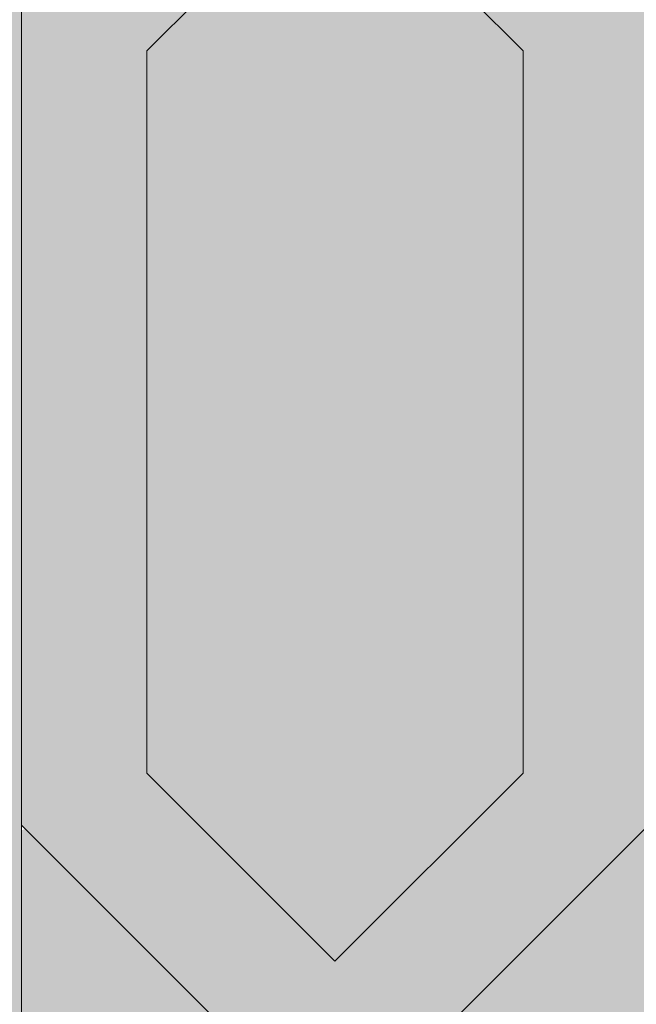
# Model space of a CAD drawing. Units: inches. Extents: x 844 to 2234, y 346 to 1084.
# Tile 78 of 93: x 1997.478 to 1998.732, y 704.51 to 706.514. Entities that reach past the tile are written whole.
import ezdxf

# ---------------------------------------------------------------- set-up
doc = ezdxf.new("R2010")
doc.units = ezdxf.units.IN
doc.header["$MEASUREMENT"] = 0
for name, color, linetype, lineweight in [('A-ANNO-DIMS', 2, 'Continuous', 18), ('furniture', 8, 'Continuous', 18), ('RA-AP-01$0$INT', 35, 'Continuous', 5)]:
    doc.layers.add(name, color=color, linetype=linetype, lineweight=lineweight)
doc.layers.add('RA-AP-01$0$FURN', color=3, linetype='Continuous')
doc.styles.get("Standard").update_dxf_attribs({"font": 'arial.ttf'})
doc.dimstyles.get("Standard").update_dxf_attribs({"dimtxt": 6, "dimasz": 3, "dimexe": 0.18, "dimexo": 0.0625, "dimgap": 0.09, "dimtad": 0, "dimtih": 1, "dimtoh": 1, "dimdec": 1, "dimzin": 0, "dimdsep": 46, "dimlunit": 3, "dimtxsty": 'Standard', "dimblk": 'ARCHTICK', "dimcen": 0.09, "dimadec": 0, "dimazin": 0, "dimtfac": 1, "dimtdec": 1, "dimtofl": 0, "dimtmove": 0, "dimatfit": 3, "dimfxl": 1, "dimtolj": 1, "dimtzin": 0, "dimarcsym": 0})

# ---------------------------------------------------------------- blocks, each defined once
blk = doc.blocks.new('A$C18D01794')
at = {"layer": 'RA-AP-01$0$INT'}
h = blk.add_hatch(color=256, dxfattribs=at)
h.paths.add_polyline_path([(4.355206456958071, -6.156712009588037), (4.355206456958071, -8.056712009588038), (5.455206456958072, -8.056712009588038), (5.455206456958072, -6.156712009588037)])
h.paths.add_polyline_path([(4.405206456958072, -8.006712009588039), (4.405206456958072, -6.206712009588038), (5.405206456958072, -6.206712009588038), (5.405206456958072, -8.006712009588039)], flags=16)
h = blk.add_hatch(color=256, dxfattribs=at)
h.paths.add_polyline_path([(4.505206456958071, -7.585498806127123), (4.46934859260189, -7.549640941759413), (4.505206456958071, -7.513783077414768), (4.505206456958071, -7.381963272220687), (4.469348592616735, -7.346105407867824), (4.505206456958071, -7.310247543514964), (4.505206456958071, -7.178427738324996), (4.469348592586679, -7.142569873965138), (4.505206456952245, -7.106712009588038), (4.476922185709333, -7.106712009588038), (4.455206456960671, -7.128427738343681), (4.433490728198047, -7.106712009588038), (4.405206456946033, -7.106712009588036), (4.441064321339216, -7.142569873969684), (4.40520645695807, -7.178427738362358), (4.405206456958072, -7.310247543472698), (4.441064321364728, -7.346105407867826), (4.40520645695807, -7.381963272262947), (4.40520645695807, -7.513783077378263), (4.441064321354429, -7.549640941786153), (4.405206456958072, -7.585498806170974), (4.405206456958072, -7.717318611286652), (4.441064321333084, -7.753176475673194), (4.405206456958072, -7.789034340036673), (4.405206456958072, -8.006712009588039), (4.644348592588106, -8.006712009588039), (4.680206456964639, -7.970854145211967), (4.716064321341165, -8.006712009588039), (4.869348592586113, -8.006712009588039), (4.905206456964143, -7.970854145210465), (4.941064321342174, -8.006712009588039), (5.094348592587118, -8.006712009588037), (5.130206456963649, -7.970854145211967), (5.166064321340178, -8.006712009588039), (5.405206456958072, -8.006712009588039), (5.405206456958072, -7.789034340024526), (5.369348592595202, -7.753176475673196), (5.40520645695807, -7.717318611298797), (5.40520645695807, -7.585498806158829), (5.369348592573859, -7.549640941786151), (5.40520645695807, -7.51378307739041), (5.40520645695807, -7.381963272250803), (5.36934859256356, -7.346105407867824), (5.405206456958072, -7.310247543484846), (5.405206456958072, -7.178427738350217), (5.369348592589068, -7.142569873969682), (5.405206456982249, -7.106712009588038), (5.376922185730244, -7.106712009588038), (5.355206456967613, -7.128427738343679), (5.333490728218955, -7.10671200958804), (5.305206456976043, -7.106712009588042), (5.341064321341609, -7.142569873965136), (5.305206456958072, -7.178427738337141), (5.305206456958072, -7.310247543502816), (5.34106432131155, -7.346105407867824), (5.305206456958072, -7.381963272232832), (5.30520645695807, -7.513783077402624), (5.341064321326395, -7.549640941759413), (5.305206456958072, -7.585498806139263), (5.305206456958072, -7.717318611299605), (5.341064321347738, -7.753176475677737), (5.305206456958072, -7.78903434007894), (5.30520645695807, -7.906712009588039), (5.166064321336834, -7.906712009588039), (5.130206456963647, -7.942569873961684), (5.094348592590464, -7.906712009588039), (4.941064321338827, -7.906712009588041), (4.905206456964145, -7.942569873963183), (4.869348592589459, -7.906712009588039), (4.716064321337822, -7.906712009588041), (4.680206456964641, -7.942569873961684), (4.644348592591453, -7.906712009588039), (4.505206456958071, -7.906712009588039), (4.505206456958071, -7.789034340066795), (4.469348592580545, -7.753176475677738), (4.505206456958071, -7.717318611311748)])
h.paths.add_polyline_path([(4.485206456974132, -7.709034340046354), (4.45520645695909, -7.739034340051736), (4.425206456974128, -7.709034340057131), (4.425206456993394, -7.593783077384998), (4.45520645699153, -7.563783077396511), (4.485206456993396, -7.593783077408017)], flags=16)
h.paths.add_polyline_path([(4.455206456954537, -7.767318611299197), (4.485206456958242, -7.797318611312542), (4.48520645695951, -7.912569873958716), (4.45520645695415, -7.942569873954422), (4.425206456957888, -7.912569873967813), (4.425206456957888, -7.797318611286197)], flags=16)
h.paths.add_polyline_path([(4.455206456964794, -7.535498806149051), (4.42520645696469, -7.5054988061393), (4.425206456983954, -7.390247543486406), (4.455206456990734, -7.360247543489279), (4.485206456983953, -7.39024754349214), (4.485206456964687, -7.505498806158811)], flags=16)
h.paths.add_polyline_path([(4.499348592588947, -7.926712009585049), (4.636064321340932, -7.926712009585049), (4.666064321342317, -7.956712009586821), (4.636064321343707, -7.986712009585048), (4.499348592575121, -7.986712009585048), (4.469348592591685, -7.956712009591957)], flags=16)
h.paths.add_polyline_path([(4.425206456957888, -7.940854145195974), (4.471064321332215, -7.986712009585049), (4.425206456957888, -7.986712009585049)], flags=16)
h.paths.add_polyline_path([(4.455206456990734, -7.331963272246367), (4.425206456989053, -7.301963272254337), (4.425206456969784, -7.186712009596224), (4.455206456965226, -7.156712009591144), (4.485206456969787, -7.186712009586051), (4.485206456989053, -7.301963272238404)], flags=16)
h.paths.add_polyline_path([(4.72434859258714, -7.926712009586255), (4.861064321340141, -7.926712009586248), (4.891064321340324, -7.956712009586823), (4.861064321340513, -7.986712009586252), (4.724348592586768, -7.986712009586252), (4.694348592586956, -7.956712009586821)], flags=16)
h.paths.add_polyline_path([(4.919348592587961, -7.956712009586821), (4.949348592588145, -7.92671200958625), (5.08606432134115, -7.926712009586253), (5.116064321341327, -7.956712009586823), (5.086064321341519, -7.986712009586252), (4.949348592587774, -7.986712009586252)], flags=16)
h.paths.add_polyline_path([(5.144348592585967, -7.956712009586823), (5.174348592587358, -7.926712009585049), (5.311064321339338, -7.926712009585049), (5.3410643213366, -7.956712009591957), (5.311064321353163, -7.986712009585048), (5.174348592584576, -7.986712009585048)], flags=16)
h.paths.add_polyline_path([(5.32520645693489, -7.593783077408021), (5.355206456936755, -7.563783077396511), (5.385206456934894, -7.593783077384998), (5.38520645695416, -7.709034340057128), (5.355206456969194, -7.739034340051736), (5.325206456954153, -7.709034340046352)], flags=16)
h.paths.add_polyline_path([(5.325206456970042, -7.797318611312542), (5.355206456973747, -7.767318611299197), (5.385206456970398, -7.7973186112862), (5.385206456970398, -7.912569873967816), (5.355206456974136, -7.942569873954422), (5.325206456968778, -7.912569873958716)], flags=16)
h.paths.add_polyline_path([(5.325206456963599, -7.505498806158811), (5.325206456944333, -7.39024754349214), (5.355206456937552, -7.360247543489279), (5.385206456944332, -7.39024754348641), (5.385206456963596, -7.505498806139303), (5.355206456963492, -7.53549880614905)], flags=16)
h.paths.add_polyline_path([(5.32520645693923, -7.301963272238403), (5.3252064569585, -7.186712009586051), (5.355206456963062, -7.156712009591142), (5.3852064569585, -7.186712009596224), (5.385206456939234, -7.301963272254338), (5.355206456937552, -7.331963272246369)], flags=16)
h.paths.add_polyline_path([(5.339348592596071, -7.986712009585048), (5.385206456970398, -7.940854145195972), (5.385206456970396, -7.986712009585048)], flags=16)
h = blk.add_hatch(color=256, dxfattribs=at)
h.paths.add_polyline_path([(4.469348592586677, -7.142569873965136), (4.505206456958073, -7.178427738324996), (4.505206456958071, -7.106712009582215)])
h.paths.add_polyline_path([(4.455206456960671, -7.128427738343681), (4.476922185709333, -7.106712009588038), (4.433490728198045, -7.106712009588038)])
h.paths.add_polyline_path([(4.405206456958073, -7.178427738362358), (4.441064321339218, -7.142569873969684), (4.40520645695807, -7.106712009600073)])
h.paths.add_polyline_path([(4.425206456989053, -7.301963272254335), (4.455206456990736, -7.331963272246371), (4.485206456989055, -7.301963272238399), (4.48520645696979, -7.186712009586054), (4.455206456965227, -7.15671200959114), (4.425206456969784, -7.186712009596224)])
h.paths.add_polyline_path([(4.505206456958073, -7.381963272220689), (4.505206456958071, -7.310247543514961), (4.469348592616738, -7.346105407867826)])
h.paths.add_polyline_path([(4.425206456964688, -7.5054988061393), (4.455206456964794, -7.535498806149051), (4.485206456964689, -7.505498806158811), (4.485206456983951, -7.390247543492138), (4.455206456990736, -7.360247543489277), (4.425206456983956, -7.39024754348641)])
h.paths.add_polyline_path([(4.425206456974126, -7.709034340057128), (4.455206456959092, -7.739034340051736), (4.485206456974132, -7.709034340046356), (4.485206456993396, -7.593783077408017), (4.45520645699153, -7.563783077396511), (4.425206456993394, -7.593783077384999)])
h.paths.add_polyline_path([(4.46934859260189, -7.549640941759415), (4.505206456958071, -7.585498806127123), (4.505206456958073, -7.513783077414766)])
h.paths.add_polyline_path([(4.405206456958073, -7.585498806170972), (4.441064321354427, -7.549640941786151), (4.405206456958072, -7.513783077378263)])
h.paths.add_polyline_path([(4.405206456958072, -7.789034340036673), (4.441064321333084, -7.753176475673194), (4.405206456958072, -7.71731861128665)])
h.paths.add_polyline_path([(4.469348592580547, -7.75317647567774), (4.505206456958071, -7.789034340066795), (4.505206456958071, -7.717318611311744)])
h.paths.add_polyline_path([(4.425206456957888, -7.912569873967814), (4.45520645695415, -7.942569873954422), (4.485206456959507, -7.912569873958718), (4.48520645695824, -7.797318611312542), (4.455206456954537, -7.767318611299197), (4.425206456957888, -7.797318611286202)])
h.paths.add_polyline_path([(4.425206456957888, -7.986712009585049), (4.471064321332215, -7.986712009585049), (4.425206456957888, -7.940854145195972)])
h.paths.add_polyline_path([(4.499348592575121, -7.986712009585048), (4.636064321343707, -7.986712009585049), (4.666064321342317, -7.956712009586823), (4.636064321340932, -7.926712009585049), (4.499348592588945, -7.926712009585049), (4.469348592591685, -7.95671200959196)])
h.paths.add_polyline_path([(4.680206456964641, -7.942569873961684), (4.716064321337824, -7.906712009588039), (4.644348592591454, -7.906712009588039)])
h.paths.add_polyline_path([(4.644348592588108, -8.006712009588039), (4.716064321341167, -8.006712009588039), (4.680206456964637, -7.970854145211964)])
h.paths.add_polyline_path([(4.724348592586768, -7.98671200958625), (4.861064321340514, -7.986712009586252), (4.891064321340324, -7.956712009586819), (4.861064321340141, -7.92671200958625), (4.724348592587134, -7.926712009586255), (4.694348592586957, -7.956712009586821)])
h.paths.add_polyline_path([(4.905206456964143, -7.942569873963183), (4.941064321338827, -7.906712009588039), (4.869348592589457, -7.906712009588037)])
h.paths.add_polyline_path([(4.869348592586113, -8.006712009588039), (4.941064321342172, -8.006712009588037), (4.905206456964145, -7.970854145210463)])
h.paths.add_polyline_path([(4.949348592587774, -7.986712009586252), (5.086064321341521, -7.986712009586252), (5.116064321341329, -7.956712009586823), (5.08606432134115, -7.926712009586253), (4.949348592588145, -7.92671200958625), (4.919348592587961, -7.956712009586819)])
h.paths.add_polyline_path([(5.130206456963645, -7.942569873961684), (5.166064321336834, -7.906712009588039), (5.094348592590464, -7.906712009588039)])
h.paths.add_polyline_path([(5.094348592587119, -8.006712009588039), (5.166064321340178, -8.006712009588039), (5.130206456963651, -7.970854145211967)])
h.paths.add_polyline_path([(5.174348592584578, -7.986712009585048), (5.311064321353163, -7.986712009585048), (5.341064321336602, -7.956712009591958), (5.31106432133934, -7.926712009585049), (5.174348592587352, -7.926712009585049), (5.144348592585969, -7.956712009586823)])
h.paths.add_polyline_path([(5.325206456968778, -7.912569873958718), (5.355206456974136, -7.942569873954422), (5.385206456970396, -7.912569873967814), (5.385206456970396, -7.797318611286199), (5.355206456973747, -7.767318611299197), (5.325206456970044, -7.797318611312544)])
h.paths.add_polyline_path([(5.339348592596073, -7.986712009585048), (5.385206456970396, -7.986712009585049), (5.385206456970398, -7.94085414519597)])
h.paths.add_polyline_path([(5.325206456954155, -7.709034340046354), (5.355206456969194, -7.739034340051734), (5.38520645695416, -7.709034340057128), (5.385206456934896, -7.593783077384999), (5.355206456936758, -7.563783077396513), (5.325206456934888, -7.593783077408019)])
h.paths.add_polyline_path([(5.305206456958072, -7.789034340078938), (5.341064321347739, -7.753176475677738), (5.305206456958072, -7.717318611299605)])
h.paths.add_polyline_path([(5.369348592595204, -7.753176475673194), (5.40520645695807, -7.789034340024526), (5.405206456958072, -7.717318611298798)])
h.paths.add_polyline_path([(5.405206456958072, -7.585498806158831), (5.405206456958072, -7.513783077390407), (5.369348592573857, -7.549640941786151)])
h.paths.add_polyline_path([(5.305206456958072, -7.585498806139266), (5.341064321326393, -7.549640941759413), (5.305206456958072, -7.513783077402626)])
h.paths.add_polyline_path([(5.325206456963599, -7.50549880615881), (5.355206456963494, -7.535498806149055), (5.385206456963598, -7.505498806139302), (5.385206456944334, -7.390247543486411), (5.355206456937552, -7.360247543489279), (5.325206456944333, -7.39024754349214)])
h.paths.add_polyline_path([(5.305206456958072, -7.38196327223283), (5.341064321311551, -7.346105407867824), (5.305206456958072, -7.31024754350282)])
h.paths.add_polyline_path([(5.325206456939231, -7.301963272238404), (5.355206456937552, -7.331963272246369), (5.385206456939235, -7.301963272254335), (5.385206456958502, -7.186712009596224), (5.355206456963061, -7.156712009591142), (5.3252064569585, -7.186712009586051)])
h.paths.add_polyline_path([(5.404581768715993, -7.381338584008926, -0.001217816984214), (5.405206456958072, -7.381112009582329), (5.405206456958072, -7.310247543484846), (5.369348592563558, -7.346105407867826)])
h.paths.add_polyline_path([(5.36934859258907, -7.142569873969684), (5.40520645695807, -7.178427738350215), (5.405206456958072, -7.106712009612218)])
h.paths.add_polyline_path([(5.355206456967613, -7.128427738343683), (5.376922185730239, -7.106712009588038), (5.333490728218953, -7.10671200958804)])
h.paths.add_polyline_path([(5.30520645695807, -7.178427738337139), (5.341064321341609, -7.142569873965134), (5.305206456958074, -7.10671200957007)])
for p, q in [((5.305206456940614, -7.381963272250288), (5.34106432131155, -7.346105407867824)), ((5.405206456940613, -7.381963272233345), (5.369348592559011, -7.346105407863277)), ((5.325206456944333, -7.39024754349214), (5.355206456937552, -7.360247543489279)), ((5.385206456944332, -7.39024754348641), (5.355206456937552, -7.360247543489279)), ((5.325206456944333, -7.39024754349214), (5.325206456963599, -7.505498806158811)), ((5.385206456944332, -7.39024754348641), (5.385206456963598, -7.5054988061393)), ((5.325206456963599, -7.505498806158811), (5.35520645696349, -7.535498806149051)), ((5.385206456963598, -7.5054988061393), (5.35520645696349, -7.535498806149051))]:
    blk.add_line(p, q, dxfattribs=at)
blk.add_lwpolyline([(5.405206456958072, -7.106712009588038), (5.405206456958072, -8.006712009588039)], dxfattribs=at)
blk = doc.blocks.new('A$C5D2F253E')
at = {"layer": 'RA-AP-01$0$FURN', "xscale": -0.7999999999883585, "yscale": 0.7999999999883585, "zscale": 0.8, "rotation": 90}
blk.add_blockref('A$C18D01794', (-5.687757199772477, 4.75791982714071), dxfattribs=at)
blk = doc.blocks.new('_ArchTick')
at = {"color": 0, "linetype": 'ByBlock', "const_width": 0.15}
blk.add_lwpolyline([(-0.5, -0.5), (0.5, 0.5)], dxfattribs=at)
blk = doc.blocks.new('*D121')
at = {"layer": 'A-ANNO-DIMS', "color": 0, "lineweight": -2, "transparency": 16777216}
for p, q in [((2030.271987351997, 734.262611118704), (2040.245275089302, 734.262611118704)), ((2040.065275089302, 734.262611118704), (2040.065275089302, 704.6043509484256)), ((2040.065275089302, 668.557359536674), (2040.065275089302, 698.2156197069523)), ((2030.271987351997, 668.557359536674), (2040.245275089302, 668.557359536674))]:
    blk.add_line(p, q, dxfattribs=at)
at = {"layer": 'Defpoints', "color": 0, "transparency": 16777216}
for p in [(2030.209487351997, 734.262611118704), (2040.065275089302, 734.262611118704), (2030.209487351997, 668.557359536674)]:
    blk.add_point(p, dxfattribs=at)
at = {"layer": 'A-ANNO-DIMS', "color": 0, "lineweight": -2, "transparency": 16777216, "xscale": 3, "yscale": 3, "zscale": 3}
for p, rotation in [((2040.065275089302, 734.262611118704), 90), ((2040.065275089302, 668.557359536674), 270)]:
    blk.add_blockref('_ArchTick', p, dxfattribs=dict(at, rotation=rotation))
at = {"layer": 'A-ANNO-DIMS', "color": 0, "transparency": 16777216, "insert": (2040.065275089302, 701.4099853276883), "char_height": 6, "attachment_point": 5}
blk.add_mtext('\\A1;LOUNGE SET 5\'-5 1/2" TYP.', dxfattribs=at)

msp = doc.modelspace()

# ---------------------------------------------------------------- block references
at = {"layer": 'furniture', "xscale": -15.94108302203742, "yscale": 15.94108302203742, "zscale": 15.94108302203742, "rotation": 270}
msp.add_blockref('A$C5D2F253E', (1990.567271852805, 701.4028671565849), dxfattribs=at)

# ---------------------------------------------------------------- dimensions: what is measured, and where the dimension line sits
at = {"layer": 'A-ANNO-DIMS'}
dim = msp.add_linear_dim(base=(2040.065275089302, 734.262611118704), p1=(2030.209487351996, 668.5573595366737), p2=(2030.209487351996, 734.2626111187037), angle=90, text='LOUNGE SET <> TYP.', dimstyle='Standard', override={"dimdec": 1, "dimlfac": 1, "dimrnd": 0, "dimzin": 1, "dimdsep": 46, "dimlunit": 4, "dimfrac": 2}, dxfattribs=at)
dim.commit()
dim.dimension.update_dxf_attribs({"geometry": '*D121', "text_midpoint": (2040.065275089302, 701.4099853276883)})

doc.saveas('drawing.dxf')
